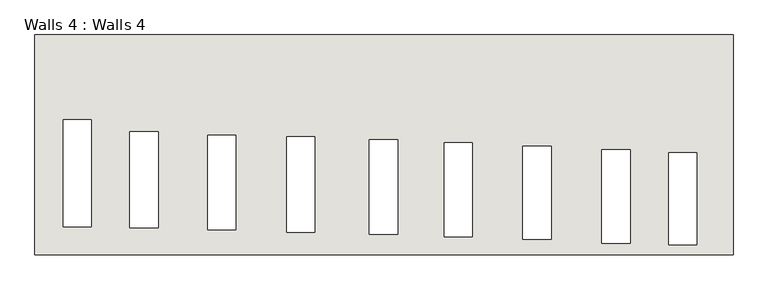
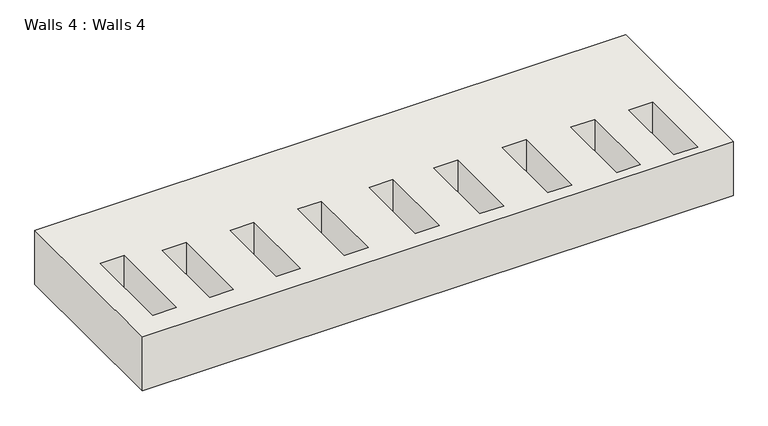
"""IFC4 building model written with IfcOpenShell, lengths in millimetres: wall geometry, Walls 4 : Walls 4."""

from ifc_helpers import new_model, si_unit, frame, origin, place, context, project, spatial, polyline, outline, extrude, source, transform, mapped, element, save


def walls_4_walls_4_fd780b34(model_context):
    return source(origin(), model_context, "Body", "SweptSolid", [
        extrude(outline(polyline([(-12951.5086202, -4306.9180898), (-12951.5086202, -3317.5420141), (-9807.4897324, -3317.5420141), (-9807.4897324, -4306.9180898), (-12951.5086202, -4306.9180898)]), holes=[polyline([(-12824.1940976, -4181.6948369), (-12697.1940976, -4181.6948369), (-12697.1940976, -3699.8487749), (-12824.1940976, -3699.8487749), (-12824.1940976, -4181.6948369)]), polyline([(-12524.0246945, -4186.5226194), (-12397.0246945, -4186.5226194), (-12397.0246945, -3752.7767395), (-12524.0246945, -3752.7767395), (-12524.0246945, -4186.5226194)]), polyline([(-12173.8270575, -4194.0735379), (-12046.8270575, -4194.0735379), (-12046.8270575, -3769.0976999), (-12173.8270575, -3769.0976999), (-12173.8270575, -4194.0735379)]), polyline([(-11818.2270575, -4205.4835161), (-11691.2270575, -4205.4835161), (-11691.2270575, -3775.5186028), (-11818.2270575, -3775.5186028), (-11818.2270575, -4205.4835161)]), polyline([(-11445.3946735, -4214.9126073), (-11318.3946735, -4214.9126073), (-11318.3946735, -3789.032782), (-11445.3946735, -3789.032782), (-11445.3946735, -4214.9126073)]), polyline([(-11109.168268, -4227.206993), (-10982.168268, -4227.206993), (-10982.168268, -3803.8263256), (-11109.168268, -3803.8263256), (-11109.168268, -4227.206993)]), polyline([(-10753.568268, -4237.3158967), (-10626.568268, -4237.3158967), (-10626.568268, -3819.285975), (-10753.568268, -3819.285975), (-10753.568268, -4237.3158967)]), polyline([(-10397.968268, -4256.1708223), (-10270.968268, -4256.1708223), (-10270.968268, -3835.082974), (-10397.968268, -3835.082974), (-10397.968268, -4256.1708223)]), polyline([(-10097.7361709, -4263.4853739), (-9970.7361709, -4263.4853739), (-9970.7361709, -3848.6675379), (-10097.7361709, -3848.6675379), (-10097.7361709, -4263.4853739)])]), frame((0.0, 0.0, 3048.0), z_axis=(0.0, 0.0, 1.0), x_axis=(1.0, 0.0, 0.0)), (0.0, 0.0, 1.0), 304.8),
    ])


if __name__ == "__main__":
    model = new_model("IFC4")
    model_context = context("Model", 3, world=origin())
    ifc_project = project(units=[si_unit("LENGTHUNIT", "METRE", prefix="MILLI")], contexts=[model_context])
    site = spatial("IfcSite", under=ifc_project)
    building = spatial("IfcBuilding", under=site)
    placement = place(None, origin())
    walls_4_walls_4_shape = walls_4_walls_4_fd780b34(model_context)
    element("IfcWall", 1, ObjectType="Walls 4 : Walls 4", at=placement, inside=building, context=model_context, shape_type="MappedRepresentation", body=[
        mapped(walls_4_walls_4_shape, transform((0.0, 0.0, 0.0), x_axis=(1.0, 0.0, 0.0), y_axis=(0.0, 1.0, 0.0), z_axis=(0.0, 0.0, 1.0))),
    ])
    save(model, "model.ifc")

# Revit data of these elements
# Element 1 (IfcWall, "Walls 4 : Walls 4")
#   Materials on its faces: "Default Wall"
# Materials
#   "Default Wall": colour RGB 80 80 80, transparency 0
